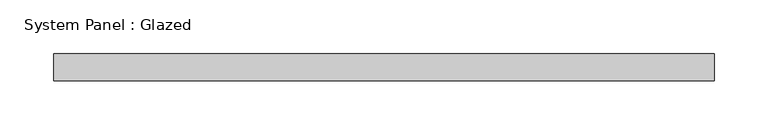
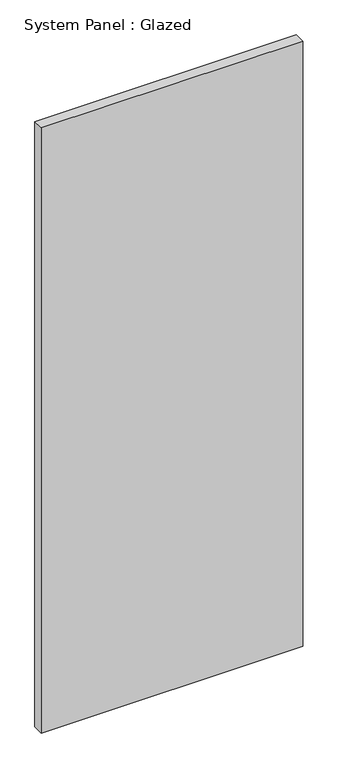
"""IFC4 building model written with IfcOpenShell, lengths in millimetres: plate geometry, System Panel : Glazed."""

from ifc_helpers import new_model, si_unit, origin, origin_with_axes, place, context, project, spatial, polyline, outline, extrude, source, transform, mapped, element, save


def system_panel_glazed_f6599d2c(model_context):
    return source(origin(), model_context, "Body", "SweptSolid", [
        extrude(outline(polyline([(307.975, 19.05), (-307.975, 19.05), (-307.975, 44.45), (307.975, 44.45), (307.975, 19.05)])), origin_with_axes(), (0.0, 0.0, 1.0), 1507.3549218),
    ])


if __name__ == "__main__":
    model = new_model("IFC4")
    model_context = context("Model", 3, world=origin())
    ifc_project = project(units=[si_unit("LENGTHUNIT", "METRE", prefix="MILLI")], contexts=[model_context])
    site = spatial("IfcSite", under=ifc_project)
    building = spatial("IfcBuilding", under=site)
    placement = place(None, origin())
    system_panel_glazed_shape = system_panel_glazed_f6599d2c(model_context)
    element("IfcPlate", 1, ObjectType="System Panel : Glazed", at=placement, inside=building, context=model_context, shape_type="MappedRepresentation", body=[
        mapped(system_panel_glazed_shape, transform((0.0, 0.0, 0.0), x_axis=(1.0, 0.0, 0.0), y_axis=(0.0, 1.0, 0.0), z_axis=(0.0, 0.0, 1.0))),
    ])
    save(model, "model.ifc")

# Revit data of these elements
# Type "System Panel : Glazed"
#   Construction Type Id = "GSP4R"
#   Analytic Construction = "1/8 in Pilkington single glazing"
#   Visual Light Transmittance = 0.9
#   Solar Heat Gain Coefficient = 0.86
#   Heat Transfer Coefficient (U) = 1.18115 BTU/(h·ft²·°F)
#   Define Thermal Properties by = 1
# Element 1 (IfcPlate, "System Panel : Glazed")
#   Materials on its faces: "Glass"
# Materials
#   "Glass": class "Glass", colour RGB 0 128 192, transparency 0.75, Description = "Soda Lime Glass", Cost = 0
